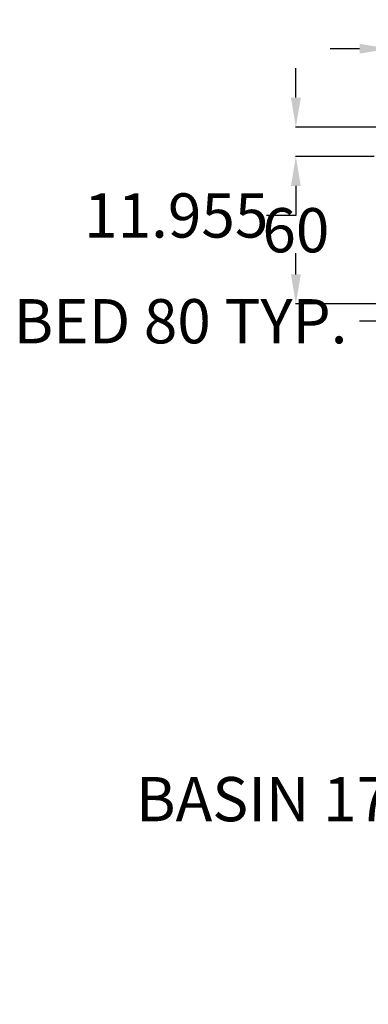
# Model space of a CAD drawing. Units: inches. Extents: x 2 to 695, y -374 to 352.
# Tile 3 of 6: x 2 to 144, y -49 to 352. Entities that reach past the tile are written whole.
import ezdxf

# ---------------------------------------------------------------- set-up
doc = ezdxf.new("R2010")
doc.units = ezdxf.units.IN
doc.layers.add('A-ANNO-DIMS', color=2, linetype='Continuous', lineweight=18)
doc.styles.get("Standard").update_dxf_attribs({"font": 'arial.ttf'})
doc.dimstyles.get("Standard").update_dxf_attribs({"dimtxt": 18, "dimasz": 12, "dimexe": 0.18, "dimexo": 0.0625, "dimgap": 0.09, "dimtad": 0, "dimtih": 1, "dimtoh": 1, "dimdec": 0, "dimzin": 0, "dimdsep": 46, "dimlunit": 3, "dimtxsty": 'Standard', "dimcen": 0.09, "dimadec": 0, "dimazin": 0, "dimtfac": 1, "dimtdec": 0, "dimtofl": 0, "dimtmove": 0, "dimatfit": 3, "dimfxl": 1, "dimtolj": 1, "dimtzin": 0, "dimarcsym": 0})

# ---------------------------------------------------------------- blocks, each defined once
blk = doc.blocks.new('*D14')
at = {"layer": 'A-ANNO-DIMS', "color": 0, "lineweight": -2, "transparency": 16777216}
for p, q in [((238.04, 37.11), (238.04, 34.48)), ((254.82, 37.11), (254.82, 34.48)), ((226.04, 34.66), (214.04, 34.66)), ((266.82, 34.66), (278.82, 34.66))]:
    blk.add_line(p, q, dxfattribs=at)
at = {"layer": 'A-ANNO-DIMS', "color": 0, "transparency": 16777216}
for points in [[(226.04, 36.66), (226.04, 32.66), (238.04, 34.66)], [(266.82, 36.66), (266.82, 32.66), (254.82, 34.66)]]:
    blk.add_solid(points, dxfattribs=at)
at = {"layer": 'Defpoints', "color": 0, "transparency": 16777216}
for p in [(238.04, 37.18), (254.82, 37.18), (238.04, 34.66)]:
    blk.add_point(p, dxfattribs=at)
at = {"layer": 'A-ANNO-DIMS', "color": 0, "transparency": 16777216, "insert": (129.31, 34.66), "char_height": 18, "attachment_point": 5}
blk.add_mtext('\\A1;BASIN 17 TYP.', dxfattribs=at)
blk = doc.blocks.new('*D16')
at = {"layer": 'A-ANNO-DIMS', "color": 0, "lineweight": -2, "transparency": 16777216}
for p, q in [((152.79, 229.15), (140.79, 229.15)), ((152.79, 217.14), (152.79, 229.33)), ((221.26, 229.15), (164.79, 229.15)), ((233.26, 217.14), (233.26, 229.33))]:
    blk.add_line(p, q, dxfattribs=at)
at = {"layer": 'A-ANNO-DIMS', "color": 0, "transparency": 16777216}
for points in [[(164.79, 231.15), (164.79, 227.15), (152.79, 229.15)], [(221.26, 231.15), (221.26, 227.15), (233.26, 229.15)]]:
    blk.add_solid(points, dxfattribs=at)
at = {"layer": 'Defpoints', "color": 0, "transparency": 16777216}
for p in [(152.79, 229.15), (152.79, 217.08), (233.26, 217.08)]:
    blk.add_point(p, dxfattribs=at)
at = {"layer": 'A-ANNO-DIMS', "color": 0, "transparency": 16777216, "insert": (67.94, 229.15), "char_height": 18, "attachment_point": 5}
blk.add_mtext('\\A1;BED 80 TYP.', dxfattribs=at)
blk = doc.blocks.new('*D33')
at = {"layer": 'A-ANNO-DIMS', "color": 0, "lineweight": -2, "transparency": 16777216}
for p, q in [((114.87, 320.13), (114.87, 332.13)), ((346.72, 308.13), (114.69, 308.13)), ((146.72, 296.18), (114.69, 296.18)), ((114.87, 284.18), (114.87, 272.18)), ((114.87, 272.18), (102.87, 272.18))]:
    blk.add_line(p, q, dxfattribs=at)
at = {"layer": 'A-ANNO-DIMS', "color": 0, "transparency": 16777216}
for points in [[(112.87, 320.13), (116.87, 320.13), (114.87, 308.13)], [(112.87, 284.18), (116.87, 284.18), (114.87, 296.18)]]:
    blk.add_solid(points, dxfattribs=at)
at = {"layer": 'Defpoints', "color": 0, "transparency": 16777216}
for p in [(346.79, 308.13), (114.87, 296.18), (146.79, 296.18)]:
    blk.add_point(p, dxfattribs=at)
at = {"layer": 'A-ANNO-DIMS', "color": 0, "transparency": 16777216, "insert": (66.2, 272.18), "char_height": 18, "attachment_point": 5}
blk.add_mtext('\\A1;11.955', dxfattribs=at)
blk = doc.blocks.new('*D34')
at = {"layer": 'A-ANNO-DIMS', "color": 0, "lineweight": -2, "transparency": 16777216}
for p, q in [((146.72, 296.18), (114.69, 296.18)), ((114.87, 284.18), (114.87, 275.46)), ((114.87, 248.18), (114.87, 256.89)), ((152.72, 236.18), (114.69, 236.18))]:
    blk.add_line(p, q, dxfattribs=at)
at = {"layer": 'A-ANNO-DIMS', "color": 0, "transparency": 16777216}
for points in [[(112.87, 284.18), (116.87, 284.18), (114.87, 296.18)], [(112.87, 248.18), (116.87, 248.18), (114.87, 236.18)]]:
    blk.add_solid(points, dxfattribs=at)
at = {"layer": 'Defpoints', "color": 0, "transparency": 16777216}
for p in [(146.79, 296.18), (114.87, 236.18), (152.79, 236.18)]:
    blk.add_point(p, dxfattribs=at)
at = {"layer": 'A-ANNO-DIMS', "color": 0, "transparency": 16777216, "insert": (114.87, 266.18), "char_height": 18, "attachment_point": 5}
blk.add_mtext('\\A1;60', dxfattribs=at)
blk = doc.blocks.new('*D40')
at = {"layer": 'A-ANNO-DIMS', "color": 0, "lineweight": -2, "transparency": 16777216}
for p, q in [((140.785845, 340.044756), (128.785845, 340.044756)), ((152.785845, 101.237546), (152.785845, 340.224756)), ((192.785845, 101.237546), (192.785845, 340.224756)), ((204.785845, 340.044756), (216.785845, 340.044756))]:
    blk.add_line(p, q, dxfattribs=at)
at = {"layer": 'A-ANNO-DIMS', "color": 0, "transparency": 16777216}
for points in [[(140.785845, 342.044756), (140.785845, 338.044756), (152.785845, 340.044756)], [(204.785845, 342.044756), (204.785845, 338.044756), (192.785845, 340.044756)]]:
    blk.add_solid(points, dxfattribs=at)
at = {"layer": 'Defpoints', "color": 0, "transparency": 16777216}
for p in [(192.785845, 340.044756), (152.785845, 101.175046), (192.785845, 101.175046)]:
    blk.add_point(p, dxfattribs=at)
at = {"layer": 'A-ANNO-DIMS', "color": 0, "transparency": 16777216, "insert": (172.785845, 340.044756), "char_height": 18, "attachment_point": 5}
blk.add_mtext('\\A1;40', dxfattribs=at)
blk = doc.blocks.new('*D46')
at = {"layer": 'A-ANNO-DIMS', "color": 0, "lineweight": -2, "transparency": 16777216}
for p, q in [((140.785845, 340.044756), (128.785845, 340.044756)), ((152.785845, -48.762454), (152.785845, 340.224756)), ((185.785845, -48.762454), (185.785845, 340.224756)), ((197.785845, 340.044756), (209.785845, 340.044756))]:
    blk.add_line(p, q, dxfattribs=at)
at = {"layer": 'A-ANNO-DIMS', "color": 0, "transparency": 16777216}
for points in [[(140.785845, 342.044756), (140.785845, 338.044756), (152.785845, 340.044756)], [(197.785845, 342.044756), (197.785845, 338.044756), (185.785845, 340.044756)]]:
    blk.add_solid(points, dxfattribs=at)
at = {"layer": 'Defpoints', "color": 0, "transparency": 16777216}
for p in [(185.785845, 340.044756), (152.785845, -48.824954), (185.785845, -48.824954)]:
    blk.add_point(p, dxfattribs=at)
at = {"layer": 'A-ANNO-DIMS', "color": 0, "transparency": 16777216, "insert": (169.285845, 340.044756), "char_height": 18, "attachment_point": 5}
blk.add_mtext('\\A1;33', dxfattribs=at)

msp = doc.modelspace()

# ---------------------------------------------------------------- dimensions: what is measured, and where the dimension line sits
at = {"layer": 'A-ANNO-DIMS'}
for base, p1, p2, picture, middle in [((192.7858, 340.0448), (152.7858, 101.175), (192.7858, 101.175), '*D40', (172.7858, 340.0448)), ((185.7858, 340.0448), (152.7858, -48.825), (185.7858, -48.825), '*D46', (169.2858, 340.0448))]:
    dim = msp.add_linear_dim(base=base, p1=p1, p2=p2, dimstyle='Standard', override={"dimdec": 0, "dimlfac": 1, "dimrnd": 0, "dimzin": 0, "dimdsep": 46, "dimlunit": 2}, dxfattribs=at)
    dim.commit()
    dim.dimension.update_dxf_attribs({"geometry": picture, "text_midpoint": middle})
for base, p1, p2, override, picture, middle in [((114.8708, 296.175), (346.7858, 308.1298), (146.7858, 296.175), {"dimdec": 3, "dimlfac": 1, "dimrnd": 0, "dimzin": 0, "dimdsep": 46, "dimlunit": 2}, '*D33', (66.1976, 272.175)), ((114.8708, 236.175), (146.7858, 296.175), (152.7858, 236.175), {"dimdec": 0, "dimlfac": 1, "dimrnd": 0, "dimzin": 0, "dimdsep": 46, "dimlunit": 2}, '*D34', (114.8708, 266.175))]:
    dim = msp.add_linear_dim(base=base, p1=p1, p2=p2, angle=90, dimstyle='Standard', override=override, dxfattribs=at)
    dim.commit()
    dim.dimension.update_dxf_attribs({"geometry": picture, "text_midpoint": middle})
for base, p1, p2, text, picture, middle in [((152.7858, 229.1519), (233.2581, 217.0811), (152.7858, 217.0811), 'BED <> TYP.', '*D16', (67.9407, 229.1519)), ((238.0373, 34.6572), (254.823, 37.175), (238.0373, 37.175), 'BASIN <> TYP.', '*D14', (129.3129, 34.6572))]:
    dim = msp.add_linear_dim(base=base, p1=p1, p2=p2, angle=180, text=text, dimstyle='Standard', override={"dimdec": 0, "dimlfac": 1, "dimrnd": 0, "dimzin": 0, "dimdsep": 46, "dimlunit": 2}, dxfattribs=at)
    dim.commit()
    dim.dimension.update_dxf_attribs({"geometry": picture, "text_midpoint": middle})

doc.saveas('drawing.dxf')
